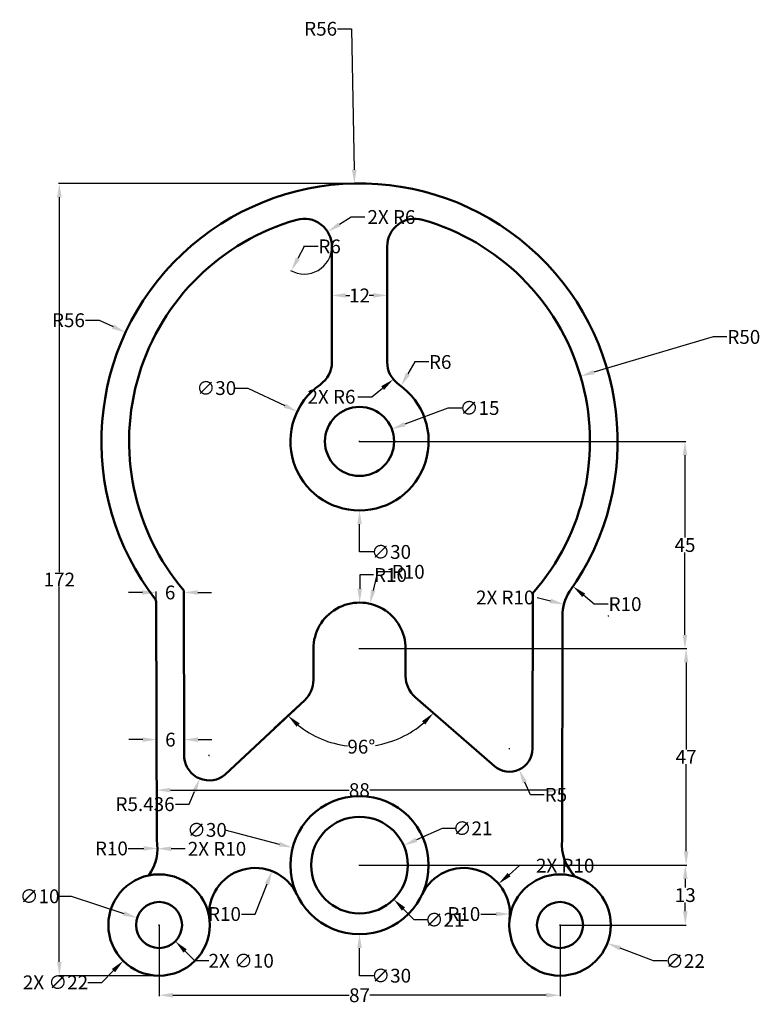
# Model space of a CAD drawing. Units: millimetres. Extents: x -15 to 146, y -9 to 205.
import ezdxf

# ---------------------------------------------------------------- set-up
doc = ezdxf.new("R2010")
doc.units = ezdxf.units.MM
doc.header["$MEASUREMENT"] = 0
doc.layers.add('M-DIMS', color=2, linetype='Continuous', lineweight=25)
doc.layers.add('M-OUTL', color=7, linetype='Continuous', lineweight=50)
doc.styles.get("Standard").update_dxf_attribs({"font": 'arial.ttf'})
doc.dimstyles.get("Standard").update_dxf_attribs({"dimtxt": 3, "dimasz": 3, "dimexe": 0.18, "dimexo": 0.0625, "dimgap": 0.09, "dimtad": 0, "dimtih": 1, "dimtoh": 1, "dimdec": 3, "dimdsep": 46, "dimtxsty": 'Standard', "dimcen": 0.09, "dimadec": 0, "dimazin": 0, "dimtfac": 1, "dimtdec": 3, "dimtofl": 0, "dimtmove": 0, "dimatfit": 3, "dimfxl": 1, "dimtolj": 1, "dimtzin": 0, "dimarcsym": 0})

# ---------------------------------------------------------------- blocks, each defined once
blk = doc.blocks.new('*D1')
at = {"layer": 'Defpoints', "color": 0, "transparency": 16777216}
for p in [(59.03, 68.42), (59.03, 68.42), (53.55, 47.86), (91.93, 39.76), (25.01, 36.5)]:
    blk.add_point(p, dxfattribs=at)
at = {"layer": 'M-DIMS', "color": 0, "lineweight": -2, "transparency": 16777216}
for start, end in [(231.26, 262.8788), (279.2658, 310.8628)]:
    blk.add_arc((59.03, 68.42), 21.28, start, end, dxfattribs=at)
at = {"layer": 'M-DIMS', "color": 0, "transparency": 16777216}
for points in [[(45.37, 51.46), (46.05, 52.19), (43.51, 53.86)], [(72.6, 52.68), (73.3, 51.97), (75.08, 54.45)]]:
    blk.add_solid(points, dxfattribs=at)
at = {"layer": 'M-DIMS', "color": 0, "transparency": 16777216, "insert": (59.42, 47.14), "char_height": 3, "attachment_point": 5}
blk.add_mtext('\\A1;96°', dxfattribs=at)
blk = doc.blocks.new('*D2')
at = {"layer": 'Defpoints', "color": 0, "transparency": 16777216}
for p in [(14.99, 40.02), (102.99, 39.88), (102.99, 37.71)]:
    blk.add_point(p, dxfattribs=at)
at = {"layer": 'M-DIMS', "color": 0, "lineweight": -2, "transparency": 16777216}
for p, q in [((14.99, 39.96), (14.99, 37.53)), ((102.99, 39.82), (102.99, 37.53)), ((17.99, 37.71), (56.75, 37.71)), ((99.99, 37.71), (61.24, 37.71))]:
    blk.add_line(p, q, dxfattribs=at)
at = {"layer": 'M-DIMS', "color": 0, "transparency": 16777216}
for points in [[(17.99, 38.21), (17.99, 37.21), (14.99, 37.71)], [(99.99, 38.21), (99.99, 37.21), (102.99, 37.71)]]:
    blk.add_solid(points, dxfattribs=at)
at = {"layer": 'M-DIMS', "color": 0, "transparency": 16777216, "insert": (58.99, 37.71), "char_height": 3, "attachment_point": 5}
blk.add_mtext('\\A1;88', dxfattribs=at)
blk = doc.blocks.new('*D3')
at = {"layer": 'Defpoints', "color": 0, "transparency": 16777216}
for p in [(15.53, 8.42), (102.53, 8.42), (102.53, -6.82)]:
    blk.add_point(p, dxfattribs=at)
at = {"layer": 'M-DIMS', "color": 0, "lineweight": -2, "transparency": 16777216}
for p, q in [((15.53, 8.36), (15.53, -7)), ((102.53, 8.36), (102.53, -7)), ((18.53, -6.82), (56.79, -6.82)), ((99.53, -6.82), (61.27, -6.82))]:
    blk.add_line(p, q, dxfattribs=at)
at = {"layer": 'M-DIMS', "color": 0, "transparency": 16777216}
for points in [[(18.53, -6.32), (18.53, -7.32), (15.53, -6.82)], [(99.53, -6.32), (99.53, -7.32), (102.53, -6.82)]]:
    blk.add_solid(points, dxfattribs=at)
at = {"layer": 'M-DIMS', "color": 0, "transparency": 16777216, "insert": (59.03, -6.82), "char_height": 3, "attachment_point": 5}
blk.add_mtext('\\A1;87', dxfattribs=at)
blk = doc.blocks.new('*D4')
at = {"layer": 'Defpoints', "color": 0, "transparency": 16777216}
for p in [(59.03, 21.42), (129.71, 21.42), (102.53, 8.42)]:
    blk.add_point(p, dxfattribs=at)
at = {"layer": 'M-DIMS', "color": 0, "lineweight": -2, "transparency": 16777216}
for p, q in [((59.09, 21.42), (129.89, 21.42)), ((129.71, 18.42), (129.71, 16.55)), ((129.71, 11.42), (129.71, 13.3)), ((102.59, 8.42), (129.89, 8.42))]:
    blk.add_line(p, q, dxfattribs=at)
at = {"layer": 'M-DIMS', "color": 0, "transparency": 16777216}
for points in [[(129.21, 18.42), (130.21, 18.42), (129.71, 21.42)], [(129.21, 11.42), (130.21, 11.42), (129.71, 8.42)]]:
    blk.add_solid(points, dxfattribs=at)
at = {"layer": 'M-DIMS', "color": 0, "transparency": 16777216, "insert": (129.71, 14.92), "char_height": 3, "attachment_point": 5}
blk.add_mtext('\\A1;13', dxfattribs=at)
blk = doc.blocks.new('*D5')
at = {"layer": 'Defpoints', "color": 0, "transparency": 16777216}
for p in [(59.03, 68.42), (129.89, 68.42), (59.03, 21.42)]:
    blk.add_point(p, dxfattribs=at)
at = {"layer": 'M-DIMS', "color": 0, "lineweight": -2, "transparency": 16777216}
for p, q in [((59.09, 68.42), (130.07, 68.42)), ((129.89, 65.42), (129.89, 46.51)), ((129.89, 24.42), (129.89, 43.33)), ((59.09, 21.42), (130.07, 21.42))]:
    blk.add_line(p, q, dxfattribs=at)
at = {"layer": 'M-DIMS', "color": 0, "transparency": 16777216}
for points in [[(129.39, 65.42), (130.39, 65.42), (129.89, 68.42)], [(129.39, 24.42), (130.39, 24.42), (129.89, 21.42)]]:
    blk.add_solid(points, dxfattribs=at)
at = {"layer": 'M-DIMS', "color": 0, "transparency": 16777216, "insert": (129.89, 44.92), "char_height": 3, "attachment_point": 5}
blk.add_mtext('\\A1;47', dxfattribs=at)
blk = doc.blocks.new('*D6')
at = {"layer": 'Defpoints', "color": 0, "transparency": 16777216}
for p in [(59.03, 113.42), (129.64, 113.42), (59.03, 68.42)]:
    blk.add_point(p, dxfattribs=at)
at = {"layer": 'M-DIMS', "color": 0, "lineweight": -2, "transparency": 16777216}
for p, q in [((59.09, 113.42), (129.82, 113.42)), ((129.64, 110.42), (129.64, 92.54)), ((129.64, 71.42), (129.64, 89.31)), ((59.09, 68.42), (129.82, 68.42))]:
    blk.add_line(p, q, dxfattribs=at)
at = {"layer": 'M-DIMS', "color": 0, "transparency": 16777216}
for points in [[(129.14, 110.42), (130.14, 110.42), (129.64, 113.42)], [(129.14, 71.42), (130.14, 71.42), (129.64, 68.42)]]:
    blk.add_solid(points, dxfattribs=at)
at = {"layer": 'M-DIMS', "color": 0, "transparency": 16777216, "insert": (129.64, 90.92), "char_height": 3, "attachment_point": 5}
blk.add_mtext('\\A1;45', dxfattribs=at)
blk = doc.blocks.new('*D7')
at = {"layer": 'Defpoints', "color": 0, "transparency": 16777216}
for p in [(14.99, 48.67), (14.99, 44.73), (20.99, 44.74)]:
    blk.add_point(p, dxfattribs=at)
at = {"layer": 'M-DIMS', "color": 0, "lineweight": -2, "transparency": 16777216}
for p, q in [((11.99, 48.67), (8.99, 48.67)), ((14.99, 44.79), (14.99, 48.85)), ((20.99, 44.8), (20.99, 48.85)), ((23.99, 48.67), (26.99, 48.67))]:
    blk.add_line(p, q, dxfattribs=at)
at = {"layer": 'M-DIMS', "color": 0, "transparency": 16777216}
for points in [[(11.99, 49.17), (11.99, 48.17), (14.99, 48.67)], [(23.99, 49.17), (23.99, 48.17), (20.99, 48.67)]]:
    blk.add_solid(points, dxfattribs=at)
at = {"layer": 'M-DIMS', "color": 0, "transparency": 16777216, "insert": (17.99, 48.67), "char_height": 3, "attachment_point": 5}
blk.add_mtext('\\A1;6', dxfattribs=at)
blk = doc.blocks.new('*D8')
at = {"layer": 'Defpoints', "color": 0, "transparency": 16777216}
for p in [(20.93, 80.62), (14.93, 78.67), (20.93, 78.68)]:
    blk.add_point(p, dxfattribs=at)
at = {"layer": 'M-DIMS', "color": 0, "lineweight": -2, "transparency": 16777216}
for p, q in [((11.93, 80.62), (8.93, 80.62)), ((14.93, 78.74), (14.93, 80.8)), ((20.93, 78.75), (20.93, 80.8)), ((23.93, 80.62), (26.93, 80.62))]:
    blk.add_line(p, q, dxfattribs=at)
at = {"layer": 'M-DIMS', "color": 0, "transparency": 16777216}
for points in [[(11.93, 81.12), (11.93, 80.12), (14.93, 80.62)], [(23.93, 81.12), (23.93, 80.12), (20.93, 80.62)]]:
    blk.add_solid(points, dxfattribs=at)
at = {"layer": 'M-DIMS', "color": 0, "transparency": 16777216, "insert": (17.93, 80.62), "char_height": 3, "attachment_point": 5}
blk.add_mtext('\\A1;6', dxfattribs=at)
blk = doc.blocks.new('*D9')
at = {"layer": 'Defpoints', "color": 0, "transparency": 16777216}
for p in [(8.26, 137.07), (59.03, 113.42)]:
    blk.add_point(p, dxfattribs=at)
at = {"layer": 'M-DIMS', "color": 0, "lineweight": -2, "transparency": 16777216}
for p, q in [((-0.46, 139.73), (2.54, 139.73)), ((2.54, 139.73), (5.54, 138.33)), ((58.94, 113.42), (59.12, 113.42)), ((59.03, 113.33), (59.03, 113.51))]:
    blk.add_line(p, q, dxfattribs=at)
at = {"layer": 'M-DIMS', "color": 0, "transparency": 16777216}
blk.add_solid([(5.75, 138.79), (5.33, 137.88), (8.26, 137.07)], dxfattribs=at)
at = {"layer": 'M-DIMS', "color": 0, "transparency": 16777216, "insert": (-4.13, 139.73), "char_height": 3, "attachment_point": 5}
blk.add_mtext('\\A1;R56', dxfattribs=at)
blk = doc.blocks.new('*D10')
at = {"layer": 'Defpoints', "color": 0, "transparency": 16777216}
for p in [(71.03, 130.66), (68.03, 125.46)]:
    blk.add_point(p, dxfattribs=at)
at = {"layer": 'M-DIMS', "color": 0, "lineweight": -2, "transparency": 16777216}
for p, q in [((71.03, 130.66), (69.53, 128.06)), ((74.03, 130.66), (71.03, 130.66))]:
    blk.add_line(p, q, dxfattribs=at)
blk.add_arc((71.03, 130.66), 6, 235.7469, 241.7189, dxfattribs=at)
at = {"layer": 'M-DIMS', "color": 0, "transparency": 16777216}
blk.add_solid([(69.09, 128.31), (69.96, 127.81), (68.03, 125.46)], dxfattribs=at)
at = {"layer": 'M-DIMS', "color": 0, "transparency": 16777216, "insert": (76.53, 130.66), "char_height": 3, "attachment_point": 5}
blk.add_mtext('\\A1;R6', dxfattribs=at)
blk = doc.blocks.new('*D11')
at = {"layer": 'Defpoints', "color": 0, "transparency": 16777216}
for p in [(53.03, 155.76), (65.03, 155.76), (65.03, 145.11)]:
    blk.add_point(p, dxfattribs=at)
at = {"layer": 'M-DIMS', "color": 0, "lineweight": -2, "transparency": 16777216}
for p, q in [((53.03, 155.69), (53.03, 144.93)), ((65.03, 155.69), (65.03, 144.93)), ((56.03, 145.11), (56.94, 145.11)), ((62.03, 145.11), (61.11, 145.11))]:
    blk.add_line(p, q, dxfattribs=at)
at = {"layer": 'M-DIMS', "color": 0, "transparency": 16777216}
for points in [[(56.03, 145.61), (56.03, 144.61), (53.03, 145.11)], [(62.03, 145.61), (62.03, 144.61), (65.03, 145.11)]]:
    blk.add_solid(points, dxfattribs=at)
at = {"layer": 'M-DIMS', "color": 0, "transparency": 16777216, "insert": (59.03, 145.11), "char_height": 3, "attachment_point": 5}
blk.add_mtext('\\A1;12', dxfattribs=at)
blk = doc.blocks.new('*D12')
at = {"layer": 'Defpoints', "color": 0, "transparency": 16777216}
for p in [(47.03, 155.76), (44.22, 150.45)]:
    blk.add_point(p, dxfattribs=at)
at = {"layer": 'M-DIMS', "color": 0, "lineweight": -2, "transparency": 16777216}
for p, q in [((47.03, 155.76), (45.62, 153.11)), ((50.03, 155.76), (47.03, 155.76))]:
    blk.add_line(p, q, dxfattribs=at)
blk.add_arc((47.03, 155.76), 6, 240.3674, 359.4032, dxfattribs=at)
at = {"layer": 'M-DIMS', "color": 0, "transparency": 16777216}
blk.add_solid([(45.18, 153.34), (46.06, 152.87), (44.22, 150.45)], dxfattribs=at)
at = {"layer": 'M-DIMS', "color": 0, "transparency": 16777216, "insert": (52.53, 155.76), "char_height": 3, "attachment_point": 5}
blk.add_mtext('\\A1;R6', dxfattribs=at)
blk = doc.blocks.new('*D13')
at = {"layer": 'Defpoints', "color": 0, "transparency": 16777216}
for p in [(45.49, 119.9), (72.56, 106.95)]:
    blk.add_point(p, dxfattribs=at)
at = {"layer": 'M-DIMS', "color": 0, "lineweight": -2, "transparency": 16777216}
for p, q in [((31.81, 125), (34.81, 125)), ((34.81, 125), (42.79, 121.19)), ((58.94, 113.42), (59.12, 113.42)), ((59.03, 113.33), (59.03, 113.51))]:
    blk.add_line(p, q, dxfattribs=at)
at = {"layer": 'M-DIMS', "color": 0, "transparency": 16777216}
blk.add_solid([(43, 121.64), (42.57, 120.74), (45.49, 119.9)], dxfattribs=at)
at = {"layer": 'M-DIMS', "color": 0, "transparency": 16777216, "insert": (27.95, 125), "char_height": 3, "attachment_point": 5}
blk.add_mtext('\\A1;∅30', dxfattribs=at)
blk = doc.blocks.new('*D14')
at = {"layer": 'Defpoints', "color": 0, "transparency": 16777216}
for p in [(66.04, 116.08), (52.01, 110.77)]:
    blk.add_point(p, dxfattribs=at)
at = {"layer": 'M-DIMS', "color": 0, "lineweight": -2, "transparency": 16777216}
for p, q in [((78.19, 120.67), (68.85, 117.14)), ((81.19, 120.67), (78.19, 120.67)), ((58.94, 113.42), (59.12, 113.42)), ((59.03, 113.33), (59.03, 113.51))]:
    blk.add_line(p, q, dxfattribs=at)
at = {"layer": 'M-DIMS', "color": 0, "transparency": 16777216}
blk.add_solid([(68.67, 117.61), (69.02, 116.67), (66.04, 116.08)], dxfattribs=at)
at = {"layer": 'M-DIMS', "color": 0, "transparency": 16777216, "insert": (85.07, 120.67), "char_height": 3, "attachment_point": 5}
blk.add_mtext('\\A1;∅15', dxfattribs=at)
blk = doc.blocks.new('*D15')
at = {"layer": 'Defpoints', "color": 0, "transparency": 16777216}
for p in [(61.3, 78.16), (59.03, 68.42)]:
    blk.add_point(p, dxfattribs=at)
at = {"layer": 'M-DIMS', "color": 0, "lineweight": -2, "transparency": 16777216}
for p, q in [((62.92, 85.11), (61.98, 81.08)), ((65.92, 85.11), (62.92, 85.11)), ((58.94, 68.42), (59.12, 68.42)), ((59.03, 68.33), (59.03, 68.51))]:
    blk.add_line(p, q, dxfattribs=at)
at = {"layer": 'M-DIMS', "color": 0, "transparency": 16777216}
blk.add_solid([(61.5, 81.2), (62.47, 80.97), (61.3, 78.16)], dxfattribs=at)
at = {"layer": 'M-DIMS', "color": 0, "transparency": 16777216, "insert": (69.59, 85.11), "char_height": 3, "attachment_point": 5}
blk.add_mtext('\\A1;R10', dxfattribs=at)
blk = doc.blocks.new('*D16')
at = {"layer": 'Defpoints', "color": 0, "transparency": 16777216}
for p in [(105.36, 81.93), (113.05, 75.54)]:
    blk.add_point(p, dxfattribs=at)
at = {"layer": 'M-DIMS', "color": 0, "lineweight": -2, "transparency": 16777216}
for p, q in [((109.97, 78.09), (107.66, 80.01)), ((112.97, 78.09), (109.97, 78.09))]:
    blk.add_line(p, q, dxfattribs=at)
blk.add_arc((113.05, 75.54), 10, 139.2564, 147.5438, dxfattribs=at)
at = {"layer": 'M-DIMS', "color": 0, "transparency": 16777216}
blk.add_solid([(107.98, 80.39), (107.35, 79.63), (105.36, 81.93)], dxfattribs=at)
at = {"layer": 'M-DIMS', "color": 0, "transparency": 16777216, "insert": (116.64, 78.09), "char_height": 3, "attachment_point": 5}
blk.add_mtext('\\A1;R10', dxfattribs=at)
blk = doc.blocks.new('*D17')
at = {"layer": 'Defpoints', "color": 0, "transparency": 16777216}
for p in [(44.51, 25.22), (73.54, 17.63)]:
    blk.add_point(p, dxfattribs=at)
at = {"layer": 'M-DIMS', "color": 0, "lineweight": -2, "transparency": 16777216}
for p, q in [((29.78, 29.07), (41.61, 25.97)), ((58.94, 21.42), (59.12, 21.42)), ((59.03, 21.33), (59.03, 21.51))]:
    blk.add_line(p, q, dxfattribs=at)
at = {"layer": 'M-DIMS', "color": 0, "transparency": 16777216}
blk.add_solid([(41.74, 26.46), (41.48, 25.49), (44.51, 25.22)], dxfattribs=at)
at = {"layer": 'M-DIMS', "color": 0, "transparency": 16777216, "insert": (25.92, 29.07), "char_height": 3, "attachment_point": 5}
blk.add_mtext('\\A1;∅30', dxfattribs=at)
blk = doc.blocks.new('*D18')
at = {"layer": 'Defpoints', "color": 0, "transparency": 16777216}
for p in [(68.62, 25.69), (49.43, 17.16)]:
    blk.add_point(p, dxfattribs=at)
at = {"layer": 'M-DIMS', "color": 0, "lineweight": -2, "transparency": 16777216}
for p, q in [((76.98, 29.41), (71.36, 26.91)), ((79.98, 29.41), (76.98, 29.41)), ((58.94, 21.42), (59.12, 21.42)), ((59.03, 21.33), (59.03, 21.51))]:
    blk.add_line(p, q, dxfattribs=at)
at = {"layer": 'M-DIMS', "color": 0, "transparency": 16777216}
blk.add_solid([(71.16, 27.37), (71.56, 26.46), (68.62, 25.69)], dxfattribs=at)
at = {"layer": 'M-DIMS', "color": 0, "transparency": 16777216, "insert": (83.56, 29.41), "char_height": 3, "attachment_point": 5}
blk.add_mtext('\\A1;∅21', dxfattribs=at)
blk = doc.blocks.new('*D19')
at = {"layer": 'Defpoints', "color": 0, "transparency": 16777216}
for p in [(5.19, 25.05), (15.19, 25.05)]:
    blk.add_point(p, dxfattribs=at)
at = {"layer": 'M-DIMS', "color": 0, "lineweight": -2, "transparency": 16777216}
blk.add_line((8.86, 25.05), (12.19, 25.05), dxfattribs=at)
at = {"layer": 'M-DIMS', "color": 0, "transparency": 16777216}
blk.add_solid([(12.19, 25.55), (12.19, 24.55), (15.19, 25.05)], dxfattribs=at)
at = {"layer": 'M-DIMS', "color": 0, "transparency": 16777216, "insert": (5.19, 25.05), "char_height": 3, "attachment_point": 5}
blk.add_mtext('\\A1;R10', dxfattribs=at)
blk = doc.blocks.new('*D20')
at = {"layer": 'Defpoints', "color": 0, "transparency": 16777216}
for p in [(40.04, 20.12), (36.39, 10.81)]:
    blk.add_point(p, dxfattribs=at)
at = {"layer": 'M-DIMS', "color": 0, "lineweight": -2, "transparency": 16777216}
for p, q in [((36.39, 10.81), (38.95, 17.33)), ((33.39, 10.81), (36.39, 10.81))]:
    blk.add_line(p, q, dxfattribs=at)
at = {"layer": 'M-DIMS', "color": 0, "transparency": 16777216}
blk.add_solid([(38.48, 17.51), (39.41, 17.15), (40.04, 20.12)], dxfattribs=at)
at = {"layer": 'M-DIMS', "color": 0, "transparency": 16777216, "insert": (29.72, 10.81), "char_height": 3, "attachment_point": 5}
blk.add_mtext('\\A1;R10', dxfattribs=at)
blk = doc.blocks.new('*D21')
at = {"layer": 'Defpoints', "color": 0, "transparency": 16777216}
for p in [(81.66, 10.81), (91.66, 10.81)]:
    blk.add_point(p, dxfattribs=at)
at = {"layer": 'M-DIMS', "color": 0, "lineweight": -2, "transparency": 16777216}
blk.add_line((85.33, 10.81), (88.66, 10.81), dxfattribs=at)
at = {"layer": 'M-DIMS', "color": 0, "transparency": 16777216}
blk.add_solid([(88.66, 11.31), (88.66, 10.31), (91.66, 10.81)], dxfattribs=at)
at = {"layer": 'M-DIMS', "color": 0, "transparency": 16777216, "insert": (81.66, 10.81), "char_height": 3, "attachment_point": 5}
blk.add_mtext('\\A1;R10', dxfattribs=at)
blk = doc.blocks.new('*D22')
at = {"layer": 'Defpoints', "color": 0, "transparency": 16777216}
for p in [(10.77, 9.98), (20.28, 6.87)]:
    blk.add_point(p, dxfattribs=at)
at = {"layer": 'M-DIMS', "color": 0, "lineweight": -2, "transparency": 16777216}
for p, q in [((-6.53, 14.66), (-3.53, 14.66)), ((-3.53, 14.66), (7.92, 10.91)), ((15.44, 8.42), (15.62, 8.42)), ((15.53, 8.33), (15.53, 8.51))]:
    blk.add_line(p, q, dxfattribs=at)
at = {"layer": 'M-DIMS', "color": 0, "transparency": 16777216}
blk.add_solid([(8.08, 11.39), (7.77, 10.44), (10.77, 9.98)], dxfattribs=at)
at = {"layer": 'M-DIMS', "color": 0, "transparency": 16777216, "insert": (-10.39, 14.66), "char_height": 3, "attachment_point": 5}
blk.add_mtext('\\A1;∅10', dxfattribs=at)
blk = doc.blocks.new('*D23')
at = {"layer": 'Defpoints', "color": 0, "transparency": 16777216}
for p in [(92.26, 12.38), (112.79, 4.47)]:
    blk.add_point(p, dxfattribs=at)
at = {"layer": 'M-DIMS', "color": 0, "lineweight": -2, "transparency": 16777216}
for p, q in [((102.44, 8.42), (102.62, 8.42)), ((102.53, 8.33), (102.53, 8.51)), ((122.78, 0.61), (115.59, 3.39)), ((125.78, 0.61), (122.78, 0.61))]:
    blk.add_line(p, q, dxfattribs=at)
at = {"layer": 'M-DIMS', "color": 0, "transparency": 16777216}
blk.add_solid([(115.77, 3.85), (115.41, 2.92), (112.79, 4.47)], dxfattribs=at)
at = {"layer": 'M-DIMS', "color": 0, "transparency": 16777216, "insert": (129.64, 0.61), "char_height": 3, "attachment_point": 5}
blk.add_mtext('\\A1;∅22', dxfattribs=at)
blk = doc.blocks.new('LUG-HOLE-D10')
for radius in [11, 5]:
    blk.add_circle((15.53, 8.42), radius)
blk = doc.blocks.new('*D25')
at = {"layer": 'Defpoints', "color": 0, "transparency": 16777216}
for p in [(-6.11, 169.41), (57.93, 169.41), (15.53, -2.58)]:
    blk.add_point(p, dxfattribs=at)
at = {"layer": 'M-DIMS', "color": 0, "lineweight": -2, "transparency": 16777216}
for p, q in [((57.86, 169.41), (-6.29, 169.41)), ((-6.11, 166.41), (-6.11, 85.02)), ((-6.11, 0.42), (-6.11, 81.82)), ((15.46, -2.58), (-6.29, -2.58))]:
    blk.add_line(p, q, dxfattribs=at)
at = {"layer": 'M-DIMS', "color": 0, "transparency": 16777216}
for points in [[(-6.61, 166.41), (-5.61, 166.41), (-6.11, 169.41)], [(-6.61, 0.42), (-5.61, 0.42), (-6.11, -2.58)]]:
    blk.add_solid(points, dxfattribs=at)
at = {"layer": 'M-DIMS', "color": 0, "transparency": 16777216, "insert": (-6.11, 83.42), "char_height": 3, "attachment_point": 5}
blk.add_mtext('\\A1;172', dxfattribs=at)
blk = doc.blocks.new('*D26')
at = {"layer": 'Defpoints', "color": 0, "transparency": 16777216}
for p in [(57.93, 169.41), (59.03, 113.42)]:
    blk.add_point(p, dxfattribs=at)
at = {"layer": 'M-DIMS', "color": 0, "lineweight": -2, "transparency": 16777216}
for p, q in [((54.27, 203.01), (57.27, 203.01)), ((57.27, 203.01), (57.87, 172.41)), ((58.94, 113.42), (59.12, 113.42)), ((59.03, 113.33), (59.03, 113.51))]:
    blk.add_line(p, q, dxfattribs=at)
at = {"layer": 'M-DIMS', "color": 0, "transparency": 16777216}
blk.add_solid([(58.37, 172.42), (57.37, 172.4), (57.93, 169.41)], dxfattribs=at)
at = {"layer": 'M-DIMS', "color": 0, "transparency": 16777216, "insert": (50.59, 203.01), "char_height": 3, "attachment_point": 5}
blk.add_mtext('\\A1;R56', dxfattribs=at)
blk = doc.blocks.new('*D27')
at = {"layer": 'Defpoints', "color": 0, "transparency": 16777216}
for p in [(106.98, 127.59), (59.03, 113.42)]:
    blk.add_point(p, dxfattribs=at)
at = {"layer": 'M-DIMS', "color": 0, "lineweight": -2, "transparency": 16777216}
for p, q in [((135.75, 136.1), (109.85, 128.45)), ((138.75, 136.1), (135.75, 136.1)), ((58.94, 113.42), (59.12, 113.42)), ((59.03, 113.33), (59.03, 113.51))]:
    blk.add_line(p, q, dxfattribs=at)
at = {"layer": 'M-DIMS', "color": 0, "transparency": 16777216}
blk.add_solid([(109.71, 128.92), (109.99, 127.97), (106.98, 127.59)], dxfattribs=at)
at = {"layer": 'M-DIMS', "color": 0, "transparency": 16777216, "insert": (142.41, 136.1), "char_height": 3, "attachment_point": 5}
blk.add_mtext('\\A1;R50', dxfattribs=at)
blk = doc.blocks.new('*D28')
at = {"layer": 'Defpoints', "color": 0, "transparency": 16777216}
for p in [(59.03, 128.42), (59.03, 98.42)]:
    blk.add_point(p, dxfattribs=at)
at = {"layer": 'M-DIMS', "color": 0, "lineweight": -2, "transparency": 16777216}
for p, q in [((58.94, 113.42), (59.12, 113.42)), ((59.03, 113.33), (59.03, 113.51)), ((59.03, 89.42), (59.03, 95.42)), ((62.03, 89.42), (59.03, 89.42))]:
    blk.add_line(p, q, dxfattribs=at)
at = {"layer": 'M-DIMS', "color": 0, "transparency": 16777216}
blk.add_solid([(59.53, 95.42), (58.53, 95.42), (59.03, 98.42)], dxfattribs=at)
at = {"layer": 'M-DIMS', "color": 0, "transparency": 16777216, "insert": (65.89, 89.42), "char_height": 3, "attachment_point": 5}
blk.add_mtext('\\A1;∅30', dxfattribs=at)
blk = doc.blocks.new('*D29')
at = {"layer": 'Defpoints', "color": 0, "transparency": 16777216}
for p in [(59.02, 36.42), (59.03, 6.42)]:
    blk.add_point(p, dxfattribs=at)
at = {"layer": 'M-DIMS', "color": 0, "lineweight": -2, "transparency": 16777216}
for p, q in [((58.94, 21.42), (59.12, 21.42)), ((59.03, 21.33), (59.03, 21.51)), ((59.03, -2.58), (59.03, 3.42)), ((62.03, -2.58), (59.03, -2.58))]:
    blk.add_line(p, q, dxfattribs=at)
at = {"layer": 'M-DIMS', "color": 0, "transparency": 16777216}
blk.add_solid([(59.53, 3.42), (58.53, 3.42), (59.03, 6.42)], dxfattribs=at)
at = {"layer": 'M-DIMS', "color": 0, "transparency": 16777216, "insert": (65.9, -2.58), "char_height": 3, "attachment_point": 5}
blk.add_mtext('\\A1;∅30', dxfattribs=at)
blk = doc.blocks.new('*D30')
at = {"layer": 'Defpoints', "color": 0, "transparency": 16777216}
for p in [(51.6, 28.85), (66.45, 14)]:
    blk.add_point(p, dxfattribs=at)
at = {"layer": 'M-DIMS', "color": 0, "lineweight": -2, "transparency": 16777216}
for p, q in [((58.94, 21.42), (59.12, 21.42)), ((59.03, 21.33), (59.03, 21.51)), ((70.91, 9.54), (68.57, 11.88)), ((73.91, 9.54), (70.91, 9.54))]:
    blk.add_line(p, q, dxfattribs=at)
at = {"layer": 'M-DIMS', "color": 0, "transparency": 16777216}
blk.add_solid([(68.93, 12.23), (68.22, 11.52), (66.45, 14)], dxfattribs=at)
at = {"layer": 'M-DIMS', "color": 0, "transparency": 16777216, "insert": (77.49, 9.54), "char_height": 3, "attachment_point": 5}
blk.add_mtext('\\A1;∅21', dxfattribs=at)
blk = doc.blocks.new('*D31')
at = {"layer": 'Defpoints', "color": 0, "transparency": 16777216}
for p in [(23.3, 16.21), (7.75, 0.64)]:
    blk.add_point(p, dxfattribs=at)
at = {"layer": 'M-DIMS', "color": 0, "lineweight": -2, "transparency": 16777216}
for p, q in [((15.44, 8.42), (15.62, 8.42)), ((15.53, 8.33), (15.53, 8.51)), ((3.09, -4.03), (5.63, -1.48)), ((0.09, -4.03), (3.09, -4.03))]:
    blk.add_line(p, q, dxfattribs=at)
at = {"layer": 'M-DIMS', "color": 0, "transparency": 16777216}
blk.add_solid([(5.28, -1.13), (5.99, -1.83), (7.75, 0.64)], dxfattribs=at)
at = {"layer": 'M-DIMS', "color": 0, "transparency": 16777216, "insert": (-6.94, -4.03), "char_height": 3, "attachment_point": 5}
blk.add_mtext('\\A1;2X ∅22', dxfattribs=at)
blk = doc.blocks.new('*D32')
at = {"layer": 'Defpoints', "color": 0, "transparency": 16777216}
for p in [(11.99, 11.95), (19.07, 4.89)]:
    blk.add_point(p, dxfattribs=at)
at = {"layer": 'M-DIMS', "color": 0, "lineweight": -2, "transparency": 16777216}
for p, q in [((15.44, 8.42), (15.62, 8.42)), ((15.53, 8.33), (15.53, 8.51)), ((23.31, 0.66), (21.19, 2.78)), ((26.31, 0.66), (23.31, 0.66))]:
    blk.add_line(p, q, dxfattribs=at)
at = {"layer": 'M-DIMS', "color": 0, "transparency": 16777216}
blk.add_solid([(21.54, 3.13), (20.84, 2.42), (19.07, 4.89)], dxfattribs=at)
at = {"layer": 'M-DIMS', "color": 0, "transparency": 16777216, "insert": (33.35, 0.66), "char_height": 3, "attachment_point": 5}
blk.add_mtext('\\A1;2X ∅10', dxfattribs=at)
blk = doc.blocks.new('*D33')
at = {"layer": 'Defpoints', "color": 0, "transparency": 16777216}
for p in [(59.06, 78.42), (59.03, 68.42)]:
    blk.add_point(p, dxfattribs=at)
at = {"layer": 'M-DIMS', "color": 0, "lineweight": -2, "transparency": 16777216}
for p, q in [((59.08, 84.42), (59.07, 81.42)), ((62.08, 84.42), (59.08, 84.42)), ((58.94, 68.42), (59.12, 68.42)), ((59.03, 68.33), (59.03, 68.51))]:
    blk.add_line(p, q, dxfattribs=at)
at = {"layer": 'M-DIMS', "color": 0, "transparency": 16777216}
blk.add_solid([(58.57, 81.43), (59.57, 81.42), (59.06, 78.42)], dxfattribs=at)
at = {"layer": 'M-DIMS', "color": 0, "transparency": 16777216, "insert": (65.75, 84.42), "char_height": 3, "attachment_point": 5}
blk.add_mtext('\\A1;R10', dxfattribs=at)
blk = doc.blocks.new('*D34')
at = {"layer": 'Defpoints', "color": 0, "transparency": 16777216}
for p in [(89.21, 17.38), (81.66, 10.81)]:
    blk.add_point(p, dxfattribs=at)
at = {"layer": 'M-DIMS', "color": 0, "lineweight": -2, "transparency": 16777216}
for p, q in [((93.73, 21.31), (91.47, 19.34)), ((96.73, 21.31), (93.73, 21.31)), ((81.57, 10.81), (81.75, 10.81)), ((81.66, 10.72), (81.66, 10.9))]:
    blk.add_line(p, q, dxfattribs=at)
at = {"layer": 'M-DIMS', "color": 0, "transparency": 16777216}
blk.add_solid([(91.14, 19.72), (91.8, 18.97), (89.21, 17.38)], dxfattribs=at)
at = {"layer": 'M-DIMS', "color": 0, "transparency": 16777216, "insert": (103.65, 21.31), "char_height": 3, "attachment_point": 5}
blk.add_mtext('\\A1;2X R10', dxfattribs=at)
blk = doc.blocks.new('*D35')
at = {"layer": 'Defpoints', "color": 0, "transparency": 16777216}
for p in [(5.19, 25.05), (15.19, 25)]:
    blk.add_point(p, dxfattribs=at)
at = {"layer": 'M-DIMS', "color": 0, "lineweight": -2, "transparency": 16777216}
for p, q in [((5.1, 25.05), (5.28, 25.05)), ((5.19, 24.96), (5.19, 25.14)), ((21.19, 24.97), (18.19, 24.98))]:
    blk.add_line(p, q, dxfattribs=at)
at = {"layer": 'M-DIMS', "color": 0, "transparency": 16777216}
blk.add_solid([(18.19, 25.48), (18.18, 24.48), (15.19, 25)], dxfattribs=at)
at = {"layer": 'M-DIMS', "color": 0, "transparency": 16777216, "insert": (28.1, 24.97), "char_height": 3, "attachment_point": 5}
blk.add_mtext('\\A1;2X R10', dxfattribs=at)
blk = doc.blocks.new('*D36')
at = {"layer": 'Defpoints', "color": 0, "transparency": 16777216}
for p in [(103.37, 78.03), (113.05, 75.54)]:
    blk.add_point(p, dxfattribs=at)
at = {"layer": 'M-DIMS', "color": 0, "lineweight": -2, "transparency": 16777216}
for p, q in [((97.56, 79.53), (100.46, 78.78)), ((112.96, 75.54), (113.14, 75.54)), ((113.05, 75.45), (113.05, 75.63))]:
    blk.add_line(p, q, dxfattribs=at)
at = {"layer": 'M-DIMS', "color": 0, "transparency": 16777216}
blk.add_solid([(100.59, 79.27), (100.34, 78.3), (103.37, 78.03)], dxfattribs=at)
at = {"layer": 'M-DIMS', "color": 0, "transparency": 16777216, "insert": (90.64, 79.53), "char_height": 3, "attachment_point": 5}
blk.add_mtext('\\A1;2X R10', dxfattribs=at)
blk = doc.blocks.new('*D37')
at = {"layer": 'Defpoints', "color": 0, "transparency": 16777216}
for p in [(52.11, 158.94), (47.03, 155.76)]:
    blk.add_point(p, dxfattribs=at)
at = {"layer": 'M-DIMS', "color": 0, "lineweight": -2, "transparency": 16777216}
for p, q in [((57.19, 162.13), (54.65, 160.54)), ((60.19, 162.13), (57.19, 162.13)), ((46.94, 155.76), (47.12, 155.76)), ((47.03, 155.67), (47.03, 155.85))]:
    blk.add_line(p, q, dxfattribs=at)
at = {"layer": 'M-DIMS', "color": 0, "transparency": 16777216}
blk.add_solid([(54.39, 160.96), (54.92, 160.11), (52.11, 158.94)], dxfattribs=at)
at = {"layer": 'M-DIMS', "color": 0, "transparency": 16777216, "insert": (65.95, 162.13), "char_height": 3, "attachment_point": 5}
blk.add_mtext('\\A1;2X R6', dxfattribs=at)
blk = doc.blocks.new('*D38')
at = {"layer": 'Defpoints', "color": 0, "transparency": 16777216}
for p in [(71.03, 130.66), (66.36, 126.89)]:
    blk.add_point(p, dxfattribs=at)
at = {"layer": 'M-DIMS', "color": 0, "lineweight": -2, "transparency": 16777216}
for p, q in [((70.94, 130.66), (71.12, 130.66)), ((71.03, 130.57), (71.03, 130.75)), ((61.69, 123.11), (64.03, 125)), ((58.69, 123.11), (61.69, 123.11))]:
    blk.add_line(p, q, dxfattribs=at)
at = {"layer": 'M-DIMS', "color": 0, "transparency": 16777216}
blk.add_solid([(63.71, 125.39), (64.34, 124.61), (66.36, 126.89)], dxfattribs=at)
at = {"layer": 'M-DIMS', "color": 0, "transparency": 16777216, "insert": (52.94, 123.11), "char_height": 3, "attachment_point": 5}
blk.add_mtext('\\A1;2X R6', dxfattribs=at)
blk = doc.blocks.new('*D39')
at = {"layer": 'Defpoints', "color": 0, "transparency": 16777216}
for p in [(26.4, 45.25), (24.35, 40.22)]:
    blk.add_point(p, dxfattribs=at)
at = {"layer": 'M-DIMS', "color": 0, "lineweight": -2, "transparency": 16777216}
for p, q in [((26.31, 45.25), (26.49, 45.25)), ((26.4, 45.16), (26.4, 45.34)), ((22.08, 34.66), (23.21, 37.44)), ((19.08, 34.66), (22.08, 34.66))]:
    blk.add_line(p, q, dxfattribs=at)
at = {"layer": 'M-DIMS', "color": 0, "transparency": 16777216}
blk.add_solid([(22.75, 37.63), (23.68, 37.25), (24.35, 40.22)], dxfattribs=at)
at = {"layer": 'M-DIMS', "color": 0, "transparency": 16777216, "insert": (12.49, 34.66), "char_height": 3, "attachment_point": 5}
blk.add_mtext('\\A1;R5.436', dxfattribs=at)
blk = doc.blocks.new('*D40')
at = {"layer": 'Defpoints', "color": 0, "transparency": 16777216}
for p in [(91.57, 46.71), (93.64, 42.16)]:
    blk.add_point(p, dxfattribs=at)
at = {"layer": 'M-DIMS', "color": 0, "lineweight": -2, "transparency": 16777216}
for p, q in [((91.48, 46.71), (91.66, 46.71)), ((91.57, 46.62), (91.57, 46.8)), ((96.12, 36.7), (94.88, 39.43)), ((99.12, 36.7), (96.12, 36.7))]:
    blk.add_line(p, q, dxfattribs=at)
at = {"layer": 'M-DIMS', "color": 0, "transparency": 16777216}
blk.add_solid([(95.33, 39.64), (94.42, 39.22), (93.64, 42.16)], dxfattribs=at)
at = {"layer": 'M-DIMS', "color": 0, "transparency": 16777216, "insert": (101.64, 36.7), "char_height": 3, "attachment_point": 5}
blk.add_mtext('\\A1;R5', dxfattribs=at)

msp = doc.modelspace()

# ---------------------------------------------------------------- linework, layer by layer
at = {"layer": 'M-OUTL'}
for p, q in [((53.0259, 130.658), (53.0259, 155.7564)), ((65.0259, 130.658), (65.0259, 155.7564)), ((20.9869, 44.7414), (20.9309, 81.0396)), ((96.568, 46.7045), (96.62, 80.4595)), ((15.0144, 26.8997), (14.9346, 78.6747)), ((102.9744, 26.8997), (103.0495, 75.553)), ((69.0259, 68.4243), (69.0259, 62.4457)), ((49.0259, 68.4006), (49.0259, 61.6391)), ((71.0853, 57.9212), (73.5054, 55.8134)), ((88.2841, 42.9418), (71.0853, 57.9212)), ((47.1315, 57.2637), (29.9082, 41.1029)), ((47.1315, 57.2637), (40.5214, 51.0614))]:
    msp.add_line(p, q, dxfattribs=at)
for centre, radius in [((59.0259, 113.4243), 7.5), ((59.0259, 21.4243), 15), ((59.0259, 21.4243), 10.5)]:
    msp.add_circle(centre, radius, dxfattribs=at)
for centre, radius, start, end in [((59.0259, 113.4243), 56, 324.432503, 217.818034), ((59.0259, 113.4243), 50, 105.82662, 220.36803), ((47.0259, 155.7564), 6, 0, 105.82662), ((71.0259, 155.7564), 6, 74.17338, 180), ((59.0259, 113.4243), 50, 318.753661, 74.17338), ((47.0259, 130.658), 6, 304.849905, 0), ((71.0259, 130.658), 6, 180, 235.150095), ((59.0259, 113.4243), 15, 124.849905, 55.150095), ((113.0494, 75.5376), 10, 147.901942, 179.911661), ((5.4394, 75.5376), 10, 18.2832, 20.793619), ((59.0259, 68.4243), 10, 359.487311, 180.135828), ((75.0259, 62.4457), 6, 180, 228.94564), ((43.0259, 61.6391), 6, 313.177077, 0), ((91.568, 46.7123), 5, 228.94564, 359.911661), ((26.3987, 45.2542), 5.436, 185.413761, 310.210466), ((5.187, 25.0497), 10, 324.167792, 10.660933), ((112.9314, 25.9725), 10, 174.67987, 224.936348), ((36.3896, 10.8131), 10, 25.115726, 186.531672), ((81.6622, 10.8131), 10, 353.468328, 154.884274)]:
    msp.add_arc(centre, radius, start, end, dxfattribs=at)

# ---------------------------------------------------------------- block references
for p in [(0, 0), (87, 0)]:
    msp.add_blockref('LUG-HOLE-D10', p, dxfattribs=at)

# ---------------------------------------------------------------- dimensions: what is measured, and where the dimension line sits
at = {"layer": 'M-DIMS'}
for center, mpoint, picture, middle in [((59.0259, 113.4243), (57.926, 169.4135), '*D26', (50.5928, 203.0071)), ((59.0259, 113.4243), (106.9758, 127.5949), '*D27', (142.4149, 136.0973)), ((59.0259, 68.4243), (59.059, 78.4243), '*D33', (65.748, 84.4243))]:
    dim = msp.add_radius_dim(center=center, mpoint=mpoint, dimstyle='Standard', override={"dimdec": 0, "dimlfac": 1, "dimrnd": 0, "dimzin": 0, "dimdsep": 46, "dimlunit": 2}, dxfattribs=at)
    dim.commit()
    dim.dimension.update_dxf_attribs({"geometry": picture, "text_midpoint": middle, "dimtype": 164})
for base, p1, p2, override, picture, middle in [((-6.1081, 169.4135), (15.5259, -2.5757), (57.9262, 169.4135), {"dimdec": 0, "dimlfac": 1, "dimrnd": 0, "dimzin": 0, "dimdsep": 46, "dimlunit": 2}, '*D25', (-6.1081, 83.4189)), ((129.6352, 113.4243), (59.0259, 68.4243), (59.0259, 113.4243), {"dimclrd": 0, "dimclre": 0, "dimclrt": 0}, '*D6', (129.6352, 90.9243))]:
    dim = msp.add_linear_dim(base=base, p1=p1, p2=p2, angle=90, dimstyle='Standard', override=override, dxfattribs=at)
    dim.commit()
    dim.dimension.update_dxf_attribs({"geometry": picture, "text_midpoint": middle})
for center, mpoint, picture, middle in [((47.0259, 155.7564), (52.1096, 158.9433), '*D37', (65.9496, 162.1302)), ((71.0259, 130.658), (66.3595, 126.8865), '*D38', (52.9367, 123.1149)), ((5.187, 25.0497), (15.1869, 24.9996), '*D35', (21.1868, 24.9695))]:
    dim = msp.add_radius_dim(center=center, mpoint=mpoint, text='2X <>', dimstyle='Standard', override={"dimdec": 0, "dimlfac": 1, "dimrnd": 0, "dimzin": 0, "dimdsep": 46, "dimlunit": 2}, dxfattribs=at)
    dim.commit()
    dim.dimension.update_dxf_attribs({"geometry": picture, "text_midpoint": middle})
at = {"layer": 'M-DIMS', "transparency": 33554610}
for center, mpoint, picture, middle in [((47.0259, 155.7564), (44.2171, 150.4544), '*D12', (52.5337, 155.7564)), ((59.0259, 113.4243), (8.261, 137.0659), '*D9', (-4.131, 139.7291)), ((71.0259, 130.658), (68.0259, 125.4619), '*D10', (76.5337, 130.658)), ((59.0259, 68.4243), (61.3009, 78.1621), '*D15', (69.5929, 85.1087)), ((113.0494, 75.5376), (105.3568, 81.9269), '*D16', (116.6415, 78.0933)), ((5.187, 25.0497), (15.187, 25.0497), '*D19', (5.187, 25.0497)), ((36.3896, 10.8131), (40.043, 20.1219), '*D20', (29.7205, 10.8131)), ((81.6622, 10.8131), (91.6622, 10.8131), '*D21', (81.6622, 10.8131))]:
    dim = msp.add_radius_dim(center=center, mpoint=mpoint, dimstyle='Standard', override={"dimclrd": 0, "dimclre": 0, "dimclrt": 0}, dxfattribs=at)
    dim.commit()
    dim.dimension.update_dxf_attribs({"geometry": picture, "text_midpoint": middle, "dimtype": 164})
for base, p1, p2, picture, middle in [((65.0259, 145.1141), (53.0259, 155.7564), (65.0259, 155.7564), '*D11', (59.0259, 145.1141)), ((20.9346, 80.6212), (14.9346, 78.6747), (20.9346, 78.684), '*D8', (17.9346, 80.6212)), ((14.9869, 48.668), (20.9869, 44.7414), (14.9869, 44.7321), '*D7', (17.9869, 48.668)), ((102.5259, -6.8245), (15.5259, 8.4243), (102.5259, 8.4243), '*D3', (59.0259, -6.8245))]:
    dim = msp.add_linear_dim(base=base, p1=p1, p2=p2, dimstyle='Standard', override={"dimclrd": 0, "dimclre": 0, "dimclrt": 0}, dxfattribs=at)
    dim.commit()
    dim.dimension.update_dxf_attribs({"geometry": picture, "text_midpoint": middle})
at = {"layer": 'M-DIMS'}
for p1, p2, picture, middle in [((59.0258, 128.4243), (59.026, 98.4243), '*D28', (65.8916, 89.4243)), ((59.0218, 36.4243), (59.03, 6.4243), '*D29', (65.898, -2.5757)), ((51.6014, 28.8491), (66.4504, 13.9996), '*D30', (77.4862, 9.5447))]:
    dim = msp.add_diameter_dim_2p(p1=p1, p2=p2, dimstyle='Standard', override={"dimdec": 0, "dimlfac": 1, "dimrnd": 0, "dimzin": 0, "dimdsep": 46, "dimlunit": 2}, dxfattribs=at)
    dim.commit()
    dim.dimension.update_dxf_attribs({"geometry": picture, "text_midpoint": middle, "dimtype": 163})
at = {"layer": 'M-DIMS', "transparency": 33554610}
for p1, p2, picture, middle in [((72.5578, 106.9523), (45.494, 119.8964), '*D13', (27.9493, 125.004)), ((52.0106, 110.772), (66.0413, 116.0767), '*D14', (85.0723, 120.6699)), ((73.5387, 17.6322), (44.5132, 25.2165), '*D17', (29.7835, 29.0653)), ((49.4328, 17.1555), (68.619, 25.6932), '*D18', (83.5573, 29.4121)), ((20.2781, 6.8697), (10.7738, 9.979), '*D22', (-10.391, 14.6569)), ((92.2622, 12.3811), (112.7896, 4.4676), '*D23', (129.6396, 0.6145))]:
    dim = msp.add_diameter_dim_2p(p1=p1, p2=p2, dimstyle='Standard', override={"dimclrd": 0, "dimclre": 0, "dimclrt": 0}, dxfattribs=at)
    dim.commit()
    dim.dimension.update_dxf_attribs({"geometry": picture, "text_midpoint": middle, "dimtype": 163})
at = {"layer": 'M-DIMS'}
for center, mpoint, picture, middle in [((113.0494, 75.5376), (103.3662, 78.0345), '*D36', (97.5562, 79.5326)), ((81.6622, 10.8131), (89.2075, 17.3758), '*D34', (103.6524, 21.3134))]:
    dim = msp.add_radius_dim(center=center, mpoint=mpoint, text='2X <>', dimstyle='Standard', override={"dimdec": 0, "dimlfac": 1, "dimrnd": 0, "dimzin": 0, "dimdsep": 46, "dimlunit": 2}, dxfattribs=at)
    dim.commit()
    dim.dimension.update_dxf_attribs({"geometry": picture, "text_midpoint": middle, "dimtype": 164})
at = {"layer": 'M-DIMS', "transparency": 33554610}
dim = msp.add_angular_dim_2l(base=(53.5533, 47.8567), line1=((59.0259, 68.4243), (91.9342, 39.7627)), line2=((59.0259, 68.4243), (25.008, 36.505)), dimstyle='Standard', override={"dimclrd": 0, "dimclre": 0, "dimclrt": 0}, dxfattribs=at)
dim.commit()
dim.dimension.update_dxf_attribs({"geometry": '*D1', "text_midpoint": (59.4201, 47.1447)})
for base, p1, p2, picture, middle in [((129.8852, 68.4243), (59.0259, 21.4243), (59.0259, 68.4243), '*D5', (129.8852, 44.9243)), ((129.7052, 21.4243), (102.5259, 8.4243), (59.0259, 21.4243), '*D4', (129.7052, 14.9243))]:
    dim = msp.add_linear_dim(base=base, p1=p1, p2=p2, angle=90, dimstyle='Standard', override={"dimclrd": 0, "dimclre": 0, "dimclrt": 0}, dxfattribs=at)
    dim.commit()
    dim.dimension.update_dxf_attribs({"geometry": picture, "text_midpoint": middle})
at = {"layer": 'M-DIMS'}
for center, mpoint, override, picture, middle in [((26.3987, 45.2542), (24.3459, 40.2207), {"dimdec": 3, "dimlfac": 1, "dimrnd": 0, "dimzin": 0, "dimdsep": 46, "dimlunit": 2}, '*D39', (12.4939, 34.665)), ((91.568, 46.7123), (93.636, 42.16), {"dimdec": 0, "dimlfac": 1, "dimrnd": 0, "dimzin": 0, "dimdsep": 46, "dimlunit": 2}, '*D40', (101.6377, 36.6972))]:
    dim = msp.add_radius_dim(center=center, mpoint=mpoint, dimstyle='Standard', override=override, dxfattribs=at)
    dim.commit()
    dim.dimension.update_dxf_attribs({"geometry": picture, "text_midpoint": middle})
at = {"layer": 'M-DIMS', "transparency": 33554610}
dim = msp.add_linear_dim(base=(102.9945, 37.7147), p1=(14.9942, 40.0196), p2=(102.9945, 39.8839), dimstyle='Standard', override={"dimclrd": 0, "dimclre": 0, "dimclrt": 0}, dxfattribs=at)
dim.commit()
dim.dimension.update_dxf_attribs({"geometry": '*D2', "text_midpoint": (58.9943, 37.7147), "dimtype": 160})
at = {"layer": 'M-DIMS'}
for p1, p2, picture, middle in [((23.2999, 16.2067), (7.752, 0.642), '*D31', (-6.9366, -4.0275)), ((11.9855, 11.955), (19.0663, 4.8937), '*D32', (33.3492, 0.6569))]:
    dim = msp.add_diameter_dim_2p(p1=p1, p2=p2, text='2X <>', dimstyle='Standard', override={"dimdec": 0, "dimlfac": 1, "dimrnd": 0, "dimzin": 0, "dimdsep": 46, "dimlunit": 2}, dxfattribs=at)
    dim.commit()
    dim.dimension.update_dxf_attribs({"geometry": picture, "text_midpoint": middle, "dimtype": 163})

doc.saveas('drawing.dxf')
